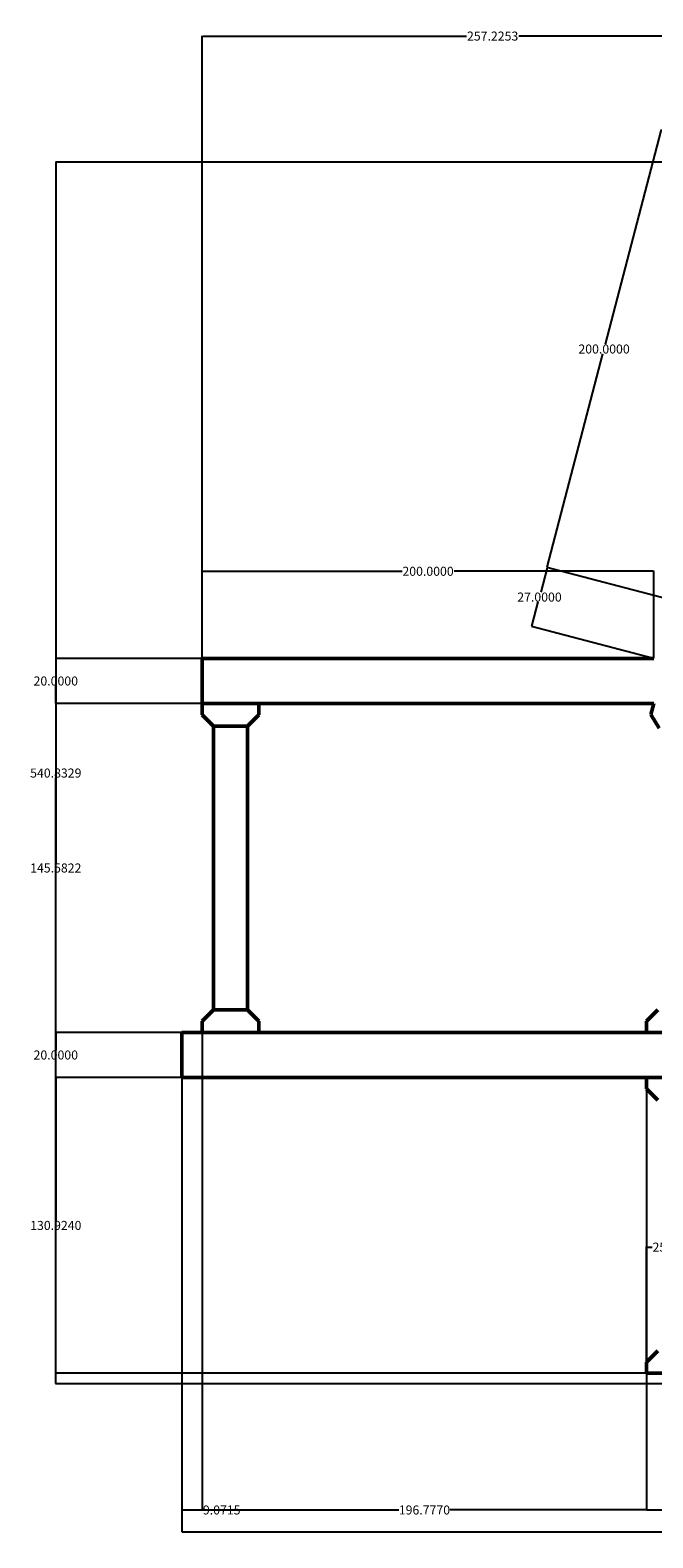
# Model space of a CAD drawing. Units: millimetres. Extents: x -54 to 1187, y -193 to 515.
# Tile 1 of 3: x -54 to 222, y -193 to 474. Entities that reach past the tile are written whole.
import ezdxf

# ---------------------------------------------------------------- set-up
doc = ezdxf.new("R2010")
doc.units = ezdxf.units.MM
doc.header["$MEASUREMENT"] = 0
doc.layers.add('M-DIMS', color=2, linetype='Continuous', lineweight=25)
doc.layers.add('M-OUTL', color=7, linetype='Continuous', lineweight=50)
doc.styles.get("Standard").update_dxf_attribs({"font": 'arial.ttf'})
doc.dimstyles.get("Standard").update_dxf_attribs({"dimtxt": 4, "dimasz": 0.18, "dimexe": 0.18, "dimexo": 0.0625, "dimgap": 0.09, "dimtad": 0, "dimtih": 1, "dimtoh": 1, "dimdec": 4, "dimzin": 0, "dimdsep": 46, "dimtxsty": 'Standard', "dimcen": 0.09, "dimclrd": 3, "dimclre": 3, "dimclrt": 1, "dimadec": 0, "dimazin": 0, "dimtfac": 1, "dimtdec": 4, "dimtofl": 0, "dimtmove": 0, "dimatfit": 3, "dimfxl": 1, "dimtolj": 1, "dimtzin": 0, "dimarcsym": 0})

# ---------------------------------------------------------------- blocks, each defined once
blk = doc.blocks.new('*D1')
at = {"layer": 'Defpoints', "color": 0, "transparency": 16777216}
for p in [(13.68, 20.33), (1113.76, 20.33), (1113.76, -190.81)]:
    blk.add_point(p, dxfattribs=at)
at = {"layer": 'M-DIMS', "color": 0, "lineweight": -2, "transparency": 16777216}
for p, q in [((13.68, 20.27), (13.68, -190.99)), ((1113.76, 20.27), (1113.76, -190.99)), ((13.86, -190.81), (550.84, -190.81)), ((1113.58, -190.81), (576.6, -190.81))]:
    blk.add_line(p, q, dxfattribs=at)
at = {"layer": 'M-DIMS', "color": 0, "transparency": 16777216}
for points in [[(13.86, -190.78), (13.86, -190.84), (13.68, -190.81)], [(1113.58, -190.78), (1113.58, -190.84), (1113.76, -190.81)]]:
    blk.add_solid(points, dxfattribs=at)
at = {"layer": 'M-DIMS', "color": 0, "transparency": 16777216, "insert": (563.72, -190.81), "char_height": 4, "attachment_point": 5}
blk.add_mtext('\\A1;1100.0835', dxfattribs=at)
blk = doc.blocks.new('*D5')
at = {"layer": 'Defpoints', "color": 0, "transparency": 16777216}
for p in [(222.75, 234.49), (22.75, 195.91), (222.75, 195.91)]:
    blk.add_point(p, dxfattribs=at)
at = {"layer": 'M-DIMS', "color": 0, "lineweight": -2, "transparency": 16777216}
for p, q in [((22.75, 195.98), (22.75, 234.67)), ((22.93, 234.49), (111.22, 234.49)), ((222.57, 234.49), (134.28, 234.49)), ((222.75, 195.98), (222.75, 234.67))]:
    blk.add_line(p, q, dxfattribs=at)
at = {"layer": 'M-DIMS', "color": 0, "transparency": 16777216}
for points in [[(22.93, 234.52), (22.93, 234.46), (22.75, 234.49)], [(222.57, 234.52), (222.57, 234.46), (222.75, 234.49)]]:
    blk.add_solid(points, dxfattribs=at)
at = {"layer": 'M-DIMS', "color": 0, "transparency": 16777216, "insert": (122.75, 234.49), "char_height": 4, "attachment_point": 5}
blk.add_mtext('\\A1;200.0000', dxfattribs=at)
blk = doc.blocks.new('*D9')
at = {"layer": 'Defpoints', "color": 0, "transparency": 16777216}
for p in [(22.75, 195.91), (-42.17, 175.91), (22.75, 175.91)]:
    blk.add_point(p, dxfattribs=at)
at = {"layer": 'M-DIMS', "color": 3, "lineweight": -2, "transparency": 16777216}
for p, q in [((22.69, 195.91), (-42.35, 195.91)), ((-42.17, 195.73), (-42.17, 188.05)), ((-42.17, 176.09), (-42.17, 183.78)), ((22.69, 175.91), (-42.35, 175.91))]:
    blk.add_line(p, q, dxfattribs=at)
at = {"layer": 'M-DIMS', "color": 3, "transparency": 16777216}
for points in [[(-42.2, 195.73), (-42.14, 195.73), (-42.17, 195.91)], [(-42.2, 176.09), (-42.14, 176.09), (-42.17, 175.91)]]:
    blk.add_solid(points, dxfattribs=at)
at = {"layer": 'M-DIMS', "color": 1, "transparency": 16777216, "insert": (-42.17, 185.91), "char_height": 4, "attachment_point": 5}
blk.add_mtext('\\A1;20.0000', dxfattribs=at)
blk = doc.blocks.new('*D10')
at = {"layer": 'Defpoints', "color": 0, "transparency": 16777216}
for p in [(22.75, 175.91), (-42.17, 30.33), (22.75, 30.33)]:
    blk.add_point(p, dxfattribs=at)
at = {"layer": 'M-DIMS', "color": 3, "lineweight": -2, "transparency": 16777216}
for p, q in [((22.69, 175.91), (-42.35, 175.91)), ((-42.17, 175.73), (-42.17, 105.25)), ((-42.17, 30.51), (-42.17, 100.99)), ((22.69, 30.33), (-42.35, 30.33))]:
    blk.add_line(p, q, dxfattribs=at)
at = {"layer": 'M-DIMS', "color": 3, "transparency": 16777216}
for points in [[(-42.2, 175.73), (-42.14, 175.73), (-42.17, 175.91)], [(-42.2, 30.51), (-42.14, 30.51), (-42.17, 30.33)]]:
    blk.add_solid(points, dxfattribs=at)
at = {"layer": 'M-DIMS', "color": 1, "transparency": 16777216, "insert": (-42.17, 103.12), "char_height": 4, "attachment_point": 5}
blk.add_mtext('\\A1;145.5822', dxfattribs=at)
blk = doc.blocks.new('*D11')
at = {"layer": 'Defpoints', "color": 0, "transparency": 16777216}
for p in [(13.68, 30.33), (-42.17, 10.33), (13.68, 10.33)]:
    blk.add_point(p, dxfattribs=at)
at = {"layer": 'M-DIMS', "color": 3, "lineweight": -2, "transparency": 16777216}
for p, q in [((13.62, 30.33), (-42.35, 30.33)), ((-42.17, 30.15), (-42.17, 22.46)), ((-42.17, 10.51), (-42.17, 18.2)), ((13.62, 10.33), (-42.35, 10.33))]:
    blk.add_line(p, q, dxfattribs=at)
at = {"layer": 'M-DIMS', "color": 3, "transparency": 16777216}
for points in [[(-42.2, 30.15), (-42.14, 30.15), (-42.17, 30.33)], [(-42.2, 10.51), (-42.14, 10.51), (-42.17, 10.33)]]:
    blk.add_solid(points, dxfattribs=at)
at = {"layer": 'M-DIMS', "color": 1, "transparency": 16777216, "insert": (-42.17, 20.33), "char_height": 4, "attachment_point": 5}
blk.add_mtext('\\A1;20.0000', dxfattribs=at)
blk = doc.blocks.new('*D12')
at = {"layer": 'Defpoints', "color": 0, "transparency": 16777216}
for p in [(219.53, 10.33), (-42.17, -120.59), (219.53, -120.59)]:
    blk.add_point(p, dxfattribs=at)
at = {"layer": 'M-DIMS', "color": 3, "lineweight": -2, "transparency": 16777216}
for p, q in [((219.46, 10.33), (-42.35, 10.33)), ((-42.17, 10.15), (-42.17, -53)), ((-42.17, -120.41), (-42.17, -57.27)), ((219.46, -120.59), (-42.35, -120.59))]:
    blk.add_line(p, q, dxfattribs=at)
at = {"layer": 'M-DIMS', "color": 3, "transparency": 16777216}
for points in [[(-42.2, 10.15), (-42.14, 10.15), (-42.17, 10.33)], [(-42.2, -120.41), (-42.14, -120.41), (-42.17, -120.59)]]:
    blk.add_solid(points, dxfattribs=at)
at = {"layer": 'M-DIMS', "color": 1, "transparency": 16777216, "insert": (-42.17, -55.13), "char_height": 4, "attachment_point": 5}
blk.add_mtext('\\A1;130.9240', dxfattribs=at)
blk = doc.blocks.new('*D13')
at = {"layer": 'Defpoints', "color": 0, "transparency": 16777216}
for p in [(-42.17, 415.58), (279.97, 415.58), (772.86, -125.25)]:
    blk.add_point(p, dxfattribs=at)
at = {"layer": 'M-DIMS', "color": 3, "lineweight": -2, "transparency": 16777216}
for p, q in [((279.91, 415.58), (-42.35, 415.58)), ((-42.17, 415.4), (-42.17, 147.3)), ((-42.17, -125.07), (-42.17, 143.03)), ((772.79, -125.25), (-42.35, -125.25))]:
    blk.add_line(p, q, dxfattribs=at)
at = {"layer": 'M-DIMS', "color": 3, "transparency": 16777216}
for points in [[(-42.2, 415.4), (-42.14, 415.4), (-42.17, 415.58)], [(-42.2, -125.07), (-42.14, -125.07), (-42.17, -125.25)]]:
    blk.add_solid(points, dxfattribs=at)
at = {"layer": 'M-DIMS', "color": 1, "transparency": 16777216, "insert": (-42.17, 145.16), "char_height": 4, "attachment_point": 5}
blk.add_mtext('\\A1;540.8329', dxfattribs=at)
blk = doc.blocks.new('*D14')
at = {"layer": 'Defpoints', "color": 0, "transparency": 16777216}
for p in [(22.75, 30.33), (13.68, 10.33), (22.75, -181.1)]:
    blk.add_point(p, dxfattribs=at)
at = {"layer": 'M-DIMS', "color": 3, "lineweight": -2, "transparency": 16777216}
for p, q in [((22.75, 30.27), (22.75, -181.28)), ((13.68, 10.27), (13.68, -181.28)), ((13.86, -181.1), (22.57, -181.1)), ((22.75, -181.1), (22.93, -181.1))]:
    blk.add_line(p, q, dxfattribs=at)
at = {"layer": 'M-DIMS', "color": 3, "transparency": 16777216}
for points in [[(13.86, -181.07), (13.86, -181.13), (13.68, -181.1)], [(22.57, -181.07), (22.57, -181.13), (22.75, -181.1)]]:
    blk.add_solid(points, dxfattribs=at)
at = {"layer": 'M-DIMS', "color": 1, "transparency": 16777216, "insert": (31.34, -181.1), "char_height": 4, "attachment_point": 5}
blk.add_mtext('\\A1;9.0715', dxfattribs=at)
blk = doc.blocks.new('*D15')
at = {"layer": 'Defpoints', "color": 0, "transparency": 16777216}
for p in [(22.75, 30.33), (219.53, 10.33), (219.53, -181.1)]:
    blk.add_point(p, dxfattribs=at)
at = {"layer": 'M-DIMS', "color": 3, "lineweight": -2, "transparency": 16777216}
for p, q in [((22.75, 30.27), (22.75, -181.28)), ((219.53, 10.27), (219.53, -181.28)), ((22.93, -181.1), (109.83, -181.1)), ((219.35, -181.1), (132.44, -181.1))]:
    blk.add_line(p, q, dxfattribs=at)
at = {"layer": 'M-DIMS', "color": 3, "transparency": 16777216}
for points in [[(22.93, -181.07), (22.93, -181.13), (22.75, -181.1)], [(219.35, -181.07), (219.35, -181.13), (219.53, -181.1)]]:
    blk.add_solid(points, dxfattribs=at)
at = {"layer": 'M-DIMS', "color": 1, "transparency": 16777216, "insert": (121.14, -181.1), "char_height": 4, "attachment_point": 5}
blk.add_mtext('\\A1;196.7770', dxfattribs=at)
blk = doc.blocks.new('*D16')
at = {"layer": 'Defpoints', "color": 0, "transparency": 16777216}
for p in [(219.53, 10.33), (404.68, 10.33), (404.68, -181.1)]:
    blk.add_point(p, dxfattribs=at)
at = {"layer": 'M-DIMS', "color": 3, "lineweight": -2, "transparency": 16777216}
for p, q in [((219.53, 10.27), (219.53, -181.28)), ((404.68, 10.27), (404.68, -181.28)), ((219.71, -181.1), (300.8, -181.1)), ((404.5, -181.1), (323.41, -181.1))]:
    blk.add_line(p, q, dxfattribs=at)
at = {"layer": 'M-DIMS', "color": 3, "transparency": 16777216}
for points in [[(219.71, -181.07), (219.71, -181.13), (219.53, -181.1)], [(404.5, -181.07), (404.5, -181.13), (404.68, -181.1)]]:
    blk.add_solid(points, dxfattribs=at)
at = {"layer": 'M-DIMS', "color": 1, "transparency": 16777216, "insert": (312.1, -181.1), "char_height": 4, "attachment_point": 5}
blk.add_mtext('\\A1;185.1524', dxfattribs=at)
blk = doc.blocks.new('*D26')
at = {"layer": 'Defpoints', "color": 0, "transparency": 16777216}
for p in [(244.53, -64.74), (219.53, -120.59), (244.53, -120.59)]:
    blk.add_point(p, dxfattribs=at)
at = {"layer": 'M-DIMS', "color": 3, "lineweight": -2, "transparency": 16777216}
for p, q in [((219.53, -120.53), (219.53, -64.56)), ((219.71, -64.74), (222.05, -64.74)), ((244.35, -64.74), (242, -64.74)), ((244.53, -120.53), (244.53, -64.56))]:
    blk.add_line(p, q, dxfattribs=at)
at = {"layer": 'M-DIMS', "color": 3, "transparency": 16777216}
for points in [[(219.71, -64.71), (219.71, -64.77), (219.53, -64.74)], [(244.35, -64.71), (244.35, -64.77), (244.53, -64.74)]]:
    blk.add_solid(points, dxfattribs=at)
at = {"layer": 'M-DIMS', "color": 1, "transparency": 16777216, "insert": (232.03, -64.74), "char_height": 4, "attachment_point": 5}
blk.add_mtext('\\A1;25.0000', dxfattribs=at)
blk = doc.blocks.new('*D28')
at = {"layer": 'Defpoints', "color": 0, "transparency": 16777216}
for p in [(279.97, 471.43), (279.97, 415.58), (22.75, 195.91)]:
    blk.add_point(p, dxfattribs=at)
at = {"layer": 'M-DIMS', "color": 3, "lineweight": -2, "transparency": 16777216}
for p, q in [((22.75, 195.98), (22.75, 471.61)), ((22.93, 471.43), (139.83, 471.43)), ((279.79, 471.43), (162.9, 471.43)), ((279.97, 415.64), (279.97, 471.61))]:
    blk.add_line(p, q, dxfattribs=at)
at = {"layer": 'M-DIMS', "color": 3, "transparency": 16777216}
for points in [[(22.93, 471.46), (22.93, 471.4), (22.75, 471.43)], [(279.79, 471.46), (279.79, 471.4), (279.97, 471.43)]]:
    blk.add_solid(points, dxfattribs=at)
at = {"layer": 'M-DIMS', "color": 1, "transparency": 16777216, "insert": (151.36, 471.43), "char_height": 4, "attachment_point": 5}
blk.add_mtext('\\A1;257.2253', dxfattribs=at)
blk = doc.blocks.new('*D30')
at = {"layer": 'Defpoints', "color": 0, "transparency": 16777216}
for p in [(225.93, 429.66), (279.97, 415.58), (229.56, 222.04)]:
    blk.add_point(p, dxfattribs=at)
at = {"layer": 'M-DIMS', "color": 3, "lineweight": -2, "transparency": 16777216}
for p, q in [((225.88, 429.49), (201.27, 335.02)), ((279.91, 415.6), (225.75, 429.71)), ((175.56, 236.29), (200.16, 330.76)), ((229.5, 222.06), (175.34, 236.17))]:
    blk.add_line(p, q, dxfattribs=at)
at = {"layer": 'M-DIMS', "color": 3, "transparency": 16777216}
for points in [[(225.85, 429.49), (225.91, 429.48), (225.93, 429.66)], [(175.53, 236.3), (175.58, 236.29), (175.51, 236.12)]]:
    blk.add_solid(points, dxfattribs=at)
at = {"layer": 'M-DIMS', "color": 1, "transparency": 16777216, "insert": (200.72, 332.89), "char_height": 4, "attachment_point": 5}
blk.add_mtext('\\A1;200.0000', dxfattribs=at)
blk = doc.blocks.new('*D37')
at = {"layer": 'Defpoints', "color": 0, "transparency": 16777216}
for p in [(175.51, 236.12), (229.56, 222.04), (222.75, 195.91)]:
    blk.add_point(p, dxfattribs=at)
at = {"layer": 'M-DIMS', "color": 3, "lineweight": -2, "transparency": 16777216}
for p, q in [((175.46, 235.95), (172.66, 225.19)), ((229.5, 222.06), (175.34, 236.17)), ((168.75, 210.17), (171.55, 220.92)), ((222.69, 195.93), (168.53, 210.04))]:
    blk.add_line(p, q, dxfattribs=at)
at = {"layer": 'M-DIMS', "color": 3, "transparency": 16777216}
for points in [[(175.44, 235.95), (175.49, 235.94), (175.51, 236.12)], [(168.72, 210.17), (168.78, 210.16), (168.7, 209.99)]]:
    blk.add_solid(points, dxfattribs=at)
at = {"layer": 'M-DIMS', "color": 1, "transparency": 16777216, "insert": (172.11, 223.06), "char_height": 4, "attachment_point": 5}
blk.add_mtext('\\A1;27.0000', dxfattribs=at)

msp = doc.modelspace()

# ---------------------------------------------------------------- linework, layer by layer
at = {"layer": 'M-OUTL'}
for p, q in [((22.74954, 175.91276), (22.74954, 195.91276)), ((22.74954, 195.91276), (222.74954, 195.91276)), ((22.74954, 175.91276), (22.74954, 170.91276)), ((22.74954, 175.91276), (222.74954, 175.91276)), ((47.74954, 170.91276), (47.74954, 175.91276)), ((222.74954, 175.91276), (221.48907, 171.07425)), ((22.74954, 170.91276), (27.74954, 165.91276)), ((47.74954, 170.91276), (42.74954, 165.91276)), ((221.48907, 171.07425), (225.06992, 164.98609)), ((27.74954, 40.33057), (27.74954, 165.91276)), ((27.74954, 165.91276), (42.74954, 165.91276)), ((42.74954, 40.33057), (42.74954, 165.91276)), ((22.74954, 35.33057), (27.74954, 40.33057)), ((27.74954, 40.33057), (42.74954, 40.33057)), ((47.74954, 35.33057), (42.74954, 40.33057)), ((219.52653, 35.33057), (224.52653, 40.33057)), ((22.74954, 30.33057), (22.74954, 35.33057)), ((47.74954, 35.33057), (47.74954, 30.33057)), ((219.52653, 30.33057), (219.52653, 35.33057)), ((13.67803, 10.33057), (13.67803, 30.33057)), ((13.67803, 30.33057), (1013.67803, 30.33057)), ((1013.67803, 10.33057), (13.67803, 10.33057)), ((219.52653, 10.33057), (219.52653, 5.33057)), ((219.52653, 5.33057), (224.52653, 0.33057)), ((219.52653, -115.5934), (224.52653, -110.5934)), ((219.52653, -120.5934), (219.52653, -115.5934)), ((219.52653, -120.5934), (244.52653, -120.5934))]:
    msp.add_line(p, q, dxfattribs=at)

# ---------------------------------------------------------------- dimensions: what is measured, and where the dimension line sits
at = {"layer": 'M-DIMS'}
for base, p1, p2, override, picture, middle in [((279.97484, 471.4313), (22.74954, 195.91276), (279.97484, 415.5813), {"dimdec": 4, "dimlfac": 1, "dimrnd": 0, "dimzin": 0, "dimdsep": 46, "dimlunit": 2}, '*D28', (151.36219, 471.4313)), ((222.74954, 234.49469), (22.74954, 195.91276), (222.74954, 195.91276), {"dimclrd": 0, "dimclre": 0, "dimclrt": 0}, '*D5', (122.74954, 234.49469)), ((22.74954, -181.10163), (13.67803, 10.33057), (22.74954, 30.33057), {"dimdec": 4, "dimlfac": 1, "dimrnd": 0, "dimzin": 0, "dimdsep": 46, "dimlunit": 2}, '*D14', (31.33741, -181.10163)), ((219.52653, -181.10163), (22.74954, 30.33057), (219.52653, 10.33057), {"dimdec": 4, "dimlfac": 1, "dimrnd": 0, "dimzin": 0, "dimdsep": 46, "dimlunit": 2}, '*D15', (121.13804, -181.10163)), ((1113.76153, -190.8134), (13.67803, 20.33057), (1113.76153, 20.33057), {"dimclrd": 0, "dimclre": 0, "dimclrt": 0}, '*D1', (563.71978, -190.8134)), ((404.67896, -181.10163), (219.52653, 10.33057), (404.67896, 10.33057), {"dimdec": 4, "dimlfac": 1, "dimrnd": 0, "dimzin": 0, "dimdsep": 46, "dimlunit": 2}, '*D16', (312.10275, -181.10163)), ((244.52653, -64.7434), (219.52653, -120.5934), (244.52653, -120.5934), {"dimdec": 4, "dimlfac": 1, "dimrnd": 0, "dimzin": 0, "dimdsep": 46, "dimlunit": 2}, '*D26', (232.02653, -64.7434))]:
    dim = msp.add_linear_dim(base=base, p1=p1, p2=p2, dimstyle='Standard', override=override, dxfattribs=at)
    dim.commit()
    dim.dimension.update_dxf_attribs({"geometry": picture, "text_midpoint": middle})
for base, p1, p2, angle, picture, middle in [((225.92864, 429.66074), (229.55607, 222.04074), (279.97484, 415.5813), 75.39855107, '*D30', (200.71925, 332.89046)), ((-42.17197, 415.5813), (772.85666, -125.25163), (279.97484, 415.5813), 90, '*D13', (-42.17197, 145.16483)), ((175.50987, 236.12018), (222.74954, 195.91276), (229.55607, 222.04074), 75.39855107, '*D37', (172.10661, 223.05619)), ((-42.17197, 175.91276), (22.74954, 195.91276), (22.74954, 175.91276), 90, '*D9', (-42.17197, 185.91276)), ((-42.17197, 30.33057), (22.74954, 175.91276), (22.74954, 30.33057), 90, '*D10', (-42.17197, 103.12167)), ((-42.17197, 10.33057), (13.67803, 30.33057), (13.67803, 10.33057), 90, '*D11', (-42.17197, 20.33057)), ((-42.17197, -120.5934), (219.52653, 10.33057), (219.52653, -120.5934), 90, '*D12', (-42.17197, -55.13142))]:
    dim = msp.add_linear_dim(base=base, p1=p1, p2=p2, angle=angle, dimstyle='Standard', override={"dimdec": 4, "dimlfac": 1, "dimrnd": 0, "dimzin": 0, "dimdsep": 46, "dimlunit": 2}, dxfattribs=at)
    dim.commit()
    dim.dimension.update_dxf_attribs({"geometry": picture, "text_midpoint": middle})

doc.saveas('drawing.dxf')
